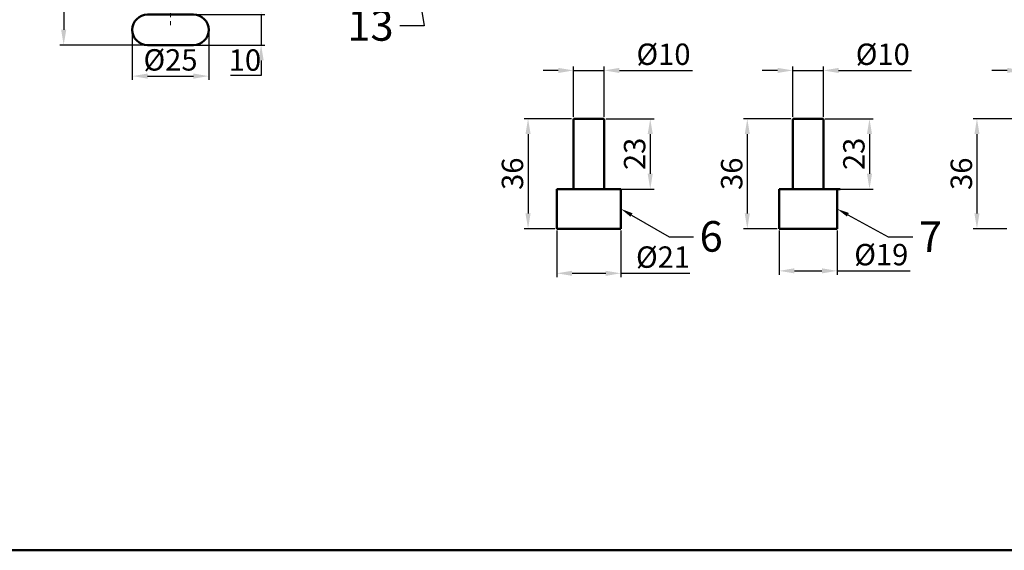
# Model space of a CAD drawing. Units: millimetres. Extents: x 434 to 1535, y -197 to 318.
# Tile 4 of 9: x 726 to 1049, y -197 to -24. Entities that reach past the tile are written whole.
import ezdxf
from ezdxf import colors
from ezdxf.entities.mleader import LeaderData, LeaderLine
from ezdxf.math import Vec2, Vec3

# ---------------------------------------------------------------- set-up
doc = ezdxf.new("R2010")
doc.units = ezdxf.units.MM
doc.header["$LTSCALE"] = 0.4
doc.linetypes.add('CENTER2', pattern=[28.575, 19.05, -3.175, 3.175, -3.175])
for name, color, linetype, lineweight in [('M-CNTR', 1, 'CENTER2', 18), ('M-DIMS', 2, 'Continuous', 25), ('M-OUTL', 7, 'Continuous', 50), ('M-TEXT', 3, 'Continuous', 25)]:
    doc.layers.add(name, color=color, linetype=linetype, lineweight=lineweight)
doc.styles.get("Standard").update_dxf_attribs({"font": 'arial.ttf'})
doc.dimstyles.new('ISO-25', dxfattribs={"dimtxt": 7, "dimasz": 5, "dimexe": 1.25, "dimexo": 0.625, "dimtad": 1, "dimtoh": 1, "dimdec": 0, "dimtxsty": 'Standard', "dimcen": 2.5, "dimadec": 0, "dimazin": 0, "dimtfac": 1, "dimtdec": 0, "dimtmove": 0, "dimatfit": 3, "dimfxl": 1, "dimarcsym": 0})

# ---------------------------------------------------------------- blocks, each defined once
blk = doc.blocks.new('*U48')
at = {"layer": 'M-CNTR', "color": 0, "transparency": 16777216}
blk.add_line((0, 223.89), (0, -74.65), dxfattribs=at)
blk = doc.blocks.new('*D53')
at = {"layer": 'Defpoints', "color": 0, "ltscale": 0.4, "transparency": 16777216}
for p in [(770.74, 232.87), (740.77, -32.13), (770.74, -32.13)]:
    blk.add_point(p, dxfattribs=at)
at = {"layer": 'M-DIMS', "color": 0, "lineweight": -2, "ltscale": 0.4, "transparency": 16777216}
for p, q in [((770.11, 232.87), (739.52, 232.87)), ((740.77, 227.87), (740.77, -27.13)), ((770.11, -32.13), (739.52, -32.13))]:
    blk.add_line(p, q, dxfattribs=at)
at = {"layer": 'M-DIMS', "color": 0, "ltscale": 0.4, "transparency": 16777216}
for points in [[(739.94, 227.87), (741.61, 227.87), (740.77, 232.87)], [(739.94, -27.13), (741.61, -27.13), (740.77, -32.13)]]:
    blk.add_solid(points, dxfattribs=at)
at = {"layer": 'M-DIMS', "color": 0, "ltscale": 0.4, "transparency": 16777216, "insert": (736.57, 100.37), "char_height": 7, "attachment_point": 5, "rotation": 90}
blk.add_mtext('265', dxfattribs=at)
blk = doc.blocks.new('*D54')
at = {"layer": 'Defpoints', "color": 0, "ltscale": 0.4, "transparency": 16777216}
for p in [(763.24, -27.13), (788.24, -27.13), (788.24, -42.28)]:
    blk.add_point(p, dxfattribs=at)
at = {"layer": 'M-DIMS', "color": 0, "lineweight": -2, "ltscale": 0.4, "transparency": 16777216}
for p, q in [((763.24, -27.75), (763.24, -43.53)), ((788.24, -27.75), (788.24, -43.53)), ((768.24, -42.28), (783.24, -42.28))]:
    blk.add_line(p, q, dxfattribs=at)
at = {"layer": 'M-DIMS', "color": 0, "ltscale": 0.4, "transparency": 16777216}
for points in [[(768.24, -41.44), (768.24, -43.11), (763.24, -42.28)], [(783.24, -41.44), (783.24, -43.11), (788.24, -42.28)]]:
    blk.add_solid(points, dxfattribs=at)
at = {"layer": 'M-DIMS', "color": 0, "ltscale": 0.4, "transparency": 16777216, "insert": (775.74, -37.88), "char_height": 7, "attachment_point": 5}
blk.add_mtext('%%C25', dxfattribs=at)
blk = doc.blocks.new('*D68')
at = {"layer": 'Defpoints', "color": 0, "ltscale": 0.4, "transparency": 16777216}
for p in [(775.74, -22.13), (775.74, -32.13), (805.39, -32.13)]:
    blk.add_point(p, dxfattribs=at)
at = {"layer": 'M-DIMS', "color": 0, "lineweight": -2, "ltscale": 0.4, "transparency": 16777216}
for p, q in [((805.39, -17.13), (805.39, -12.13)), ((776.36, -22.13), (806.64, -22.13)), ((805.39, -22.13), (805.39, -32.13)), ((776.36, -32.13), (806.64, -32.13)), ((805.39, -37.13), (805.39, -42.13)), ((805.39, -42.13), (795.42, -42.13))]:
    blk.add_line(p, q, dxfattribs=at)
at = {"layer": 'M-DIMS', "color": 0, "ltscale": 0.4, "transparency": 16777216}
for points in [[(804.55, -17.13), (806.22, -17.13), (805.39, -22.13)], [(804.55, -37.13), (806.22, -37.13), (805.39, -32.13)]]:
    blk.add_solid(points, dxfattribs=at)
at = {"layer": 'M-DIMS', "color": 0, "ltscale": 0.4, "transparency": 16777216, "insert": (800.09, -37.93), "char_height": 7, "attachment_point": 5}
blk.add_mtext('10', dxfattribs=at)
blk = doc.blocks.new('*D111')
at = {"layer": 'Defpoints', "color": 0, "ltscale": 0.4, "transparency": 16777216}
for p in [(917.65, -40.42), (907.65, -56.24), (917.65, -56.24)]:
    blk.add_point(p, dxfattribs=at)
at = {"layer": 'M-DIMS', "color": 0, "lineweight": -2, "ltscale": 0.4, "transparency": 16777216}
for p, q in [((902.65, -40.42), (897.65, -40.42)), ((907.65, -55.61), (907.65, -39.17)), ((907.65, -40.42), (917.65, -40.42)), ((917.65, -55.61), (917.65, -39.17)), ((922.65, -40.42), (946.52, -40.42))]:
    blk.add_line(p, q, dxfattribs=at)
at = {"layer": 'M-DIMS', "color": 0, "ltscale": 0.4, "transparency": 16777216}
for points in [[(902.65, -39.59), (902.65, -41.26), (907.65, -40.42)], [(922.65, -39.59), (922.65, -41.26), (917.65, -40.42)]]:
    blk.add_solid(points, dxfattribs=at)
at = {"layer": 'M-DIMS', "color": 0, "ltscale": 0.4, "transparency": 16777216, "insert": (937.08, -36.03), "char_height": 7, "attachment_point": 5}
blk.add_mtext('%%C10', dxfattribs=at)
blk = doc.blocks.new('*D112')
at = {"layer": 'Defpoints', "color": 0, "ltscale": 0.4, "transparency": 16777216}
for p in [(902.15, -92.24), (923.15, -92.24), (923.15, -106.82)]:
    blk.add_point(p, dxfattribs=at)
at = {"layer": 'M-DIMS', "color": 0, "lineweight": -2, "ltscale": 0.4, "transparency": 16777216}
for p, q in [((902.15, -92.86), (902.15, -108.07)), ((923.15, -92.86), (923.15, -108.07)), ((907.15, -106.82), (918.15, -106.82)), ((923.15, -106.82), (945.69, -106.82))]:
    blk.add_line(p, q, dxfattribs=at)
at = {"layer": 'M-DIMS', "color": 0, "ltscale": 0.4, "transparency": 16777216}
for points in [[(907.15, -105.99), (907.15, -107.66), (902.15, -106.82)], [(918.15, -105.99), (918.15, -107.66), (923.15, -106.82)]]:
    blk.add_solid(points, dxfattribs=at)
at = {"layer": 'M-DIMS', "color": 0, "ltscale": 0.4, "transparency": 16777216, "insert": (936.92, -102.43), "char_height": 7, "attachment_point": 5}
blk.add_mtext('%%C21', dxfattribs=at)
blk = doc.blocks.new('*D113')
at = {"layer": 'Defpoints', "color": 0, "ltscale": 0.4, "transparency": 16777216}
for p in [(917.65, -56.24), (917.65, -79.24), (932.74, -79.24)]:
    blk.add_point(p, dxfattribs=at)
at = {"layer": 'M-DIMS', "color": 0, "lineweight": -2, "ltscale": 0.4, "transparency": 16777216}
for p, q in [((918.27, -56.24), (933.99, -56.24)), ((932.74, -61.24), (932.74, -74.24)), ((918.27, -79.24), (933.99, -79.24))]:
    blk.add_line(p, q, dxfattribs=at)
at = {"layer": 'M-DIMS', "color": 0, "ltscale": 0.4, "transparency": 16777216}
for points in [[(931.9, -61.24), (933.57, -61.24), (932.74, -56.24)], [(931.9, -74.24), (933.57, -74.24), (932.74, -79.24)]]:
    blk.add_solid(points, dxfattribs=at)
at = {"layer": 'M-DIMS', "color": 0, "ltscale": 0.4, "transparency": 16777216, "insert": (928.54, -67.74), "char_height": 7, "attachment_point": 5, "rotation": 90}
blk.add_mtext('23', dxfattribs=at)
blk = doc.blocks.new('*D114')
at = {"layer": 'Defpoints', "color": 0, "ltscale": 0.4, "transparency": 16777216}
for p in [(907.65, -56.24), (892.75, -92.24), (902.15, -92.24)]:
    blk.add_point(p, dxfattribs=at)
at = {"layer": 'M-DIMS', "color": 0, "lineweight": -2, "ltscale": 0.4, "transparency": 16777216}
for p, q in [((907.02, -56.24), (891.5, -56.24)), ((892.75, -61.24), (892.75, -87.24)), ((901.52, -92.24), (891.5, -92.24))]:
    blk.add_line(p, q, dxfattribs=at)
at = {"layer": 'M-DIMS', "color": 0, "ltscale": 0.4, "transparency": 16777216}
for points in [[(891.91, -61.24), (893.58, -61.24), (892.75, -56.24)], [(891.91, -87.24), (893.58, -87.24), (892.75, -92.24)]]:
    blk.add_solid(points, dxfattribs=at)
at = {"layer": 'M-DIMS', "color": 0, "ltscale": 0.4, "transparency": 16777216, "insert": (888.55, -74.24), "char_height": 7, "attachment_point": 5, "rotation": 90}
blk.add_mtext('36', dxfattribs=at)
blk = doc.blocks.new('*D116')
at = {"layer": 'Defpoints', "color": 0, "ltscale": 0.4, "transparency": 16777216}
for p in [(989.4, -40.42), (979.4, -56.24), (989.4, -56.24)]:
    blk.add_point(p, dxfattribs=at)
at = {"layer": 'M-DIMS', "color": 0, "lineweight": -2, "ltscale": 0.4, "transparency": 16777216}
for p, q in [((974.4, -40.42), (969.4, -40.42)), ((979.4, -55.61), (979.4, -39.17)), ((979.4, -40.42), (989.4, -40.42)), ((989.4, -55.61), (989.4, -39.17)), ((994.4, -40.42), (1018.27, -40.42))]:
    blk.add_line(p, q, dxfattribs=at)
at = {"layer": 'M-DIMS', "color": 0, "ltscale": 0.4, "transparency": 16777216}
for points in [[(974.4, -39.59), (974.4, -41.26), (979.4, -40.42)], [(994.4, -39.59), (994.4, -41.26), (989.4, -40.42)]]:
    blk.add_solid(points, dxfattribs=at)
at = {"layer": 'M-DIMS', "color": 0, "ltscale": 0.4, "transparency": 16777216, "insert": (1008.84, -36.03), "char_height": 7, "attachment_point": 5}
blk.add_mtext('%%C10', dxfattribs=at)
blk = doc.blocks.new('*D117')
at = {"layer": 'Defpoints', "color": 0, "ltscale": 0.4, "transparency": 16777216}
for p in [(989.4, -56.24), (989.4, -79.24), (1004.49, -79.24)]:
    blk.add_point(p, dxfattribs=at)
at = {"layer": 'M-DIMS', "color": 0, "lineweight": -2, "ltscale": 0.4, "transparency": 16777216}
for p, q in [((990.03, -56.24), (1005.74, -56.24)), ((1004.49, -61.24), (1004.49, -74.24)), ((990.03, -79.24), (1005.74, -79.24))]:
    blk.add_line(p, q, dxfattribs=at)
at = {"layer": 'M-DIMS', "color": 0, "ltscale": 0.4, "transparency": 16777216}
for points in [[(1003.66, -61.24), (1005.32, -61.24), (1004.49, -56.24)], [(1003.66, -74.24), (1005.32, -74.24), (1004.49, -79.24)]]:
    blk.add_solid(points, dxfattribs=at)
at = {"layer": 'M-DIMS', "color": 0, "ltscale": 0.4, "transparency": 16777216, "insert": (1000.29, -67.74), "char_height": 7, "attachment_point": 5, "rotation": 90}
blk.add_mtext('23', dxfattribs=at)
blk = doc.blocks.new('*D115')
at = {"layer": 'Defpoints', "color": 0, "ltscale": 0.4, "transparency": 16777216}
for p in [(979.4, -56.24), (964.5, -92.24), (974.9, -92.24)]:
    blk.add_point(p, dxfattribs=at)
at = {"layer": 'M-DIMS', "color": 0, "lineweight": -2, "ltscale": 0.4, "transparency": 16777216}
for p, q in [((978.78, -56.24), (963.25, -56.24)), ((964.5, -61.24), (964.5, -87.24)), ((974.28, -92.24), (963.25, -92.24))]:
    blk.add_line(p, q, dxfattribs=at)
at = {"layer": 'M-DIMS', "color": 0, "ltscale": 0.4, "transparency": 16777216}
for points in [[(963.67, -61.24), (965.33, -61.24), (964.5, -56.24)], [(963.67, -87.24), (965.33, -87.24), (964.5, -92.24)]]:
    blk.add_solid(points, dxfattribs=at)
at = {"layer": 'M-DIMS', "color": 0, "ltscale": 0.4, "transparency": 16777216, "insert": (960.3, -74.24), "char_height": 7, "attachment_point": 5, "rotation": 90}
blk.add_mtext('36', dxfattribs=at)
blk = doc.blocks.new('*D118')
at = {"layer": 'Defpoints', "color": 0, "ltscale": 0.4, "transparency": 16777216}
for p in [(974.9, -92.24), (993.9, -92.24), (993.9, -106.02)]:
    blk.add_point(p, dxfattribs=at)
at = {"layer": 'M-DIMS', "color": 0, "lineweight": -2, "ltscale": 0.4, "transparency": 16777216}
for p, q in [((974.9, -92.86), (974.9, -107.27)), ((993.9, -92.86), (993.9, -107.27)), ((979.9, -106.02), (988.9, -106.02)), ((993.9, -106.02), (1017.81, -106.02))]:
    blk.add_line(p, q, dxfattribs=at)
at = {"layer": 'M-DIMS', "color": 0, "ltscale": 0.4, "transparency": 16777216}
for points in [[(979.9, -105.18), (979.9, -106.85), (974.9, -106.02)], [(988.9, -105.18), (988.9, -106.85), (993.9, -106.02)]]:
    blk.add_solid(points, dxfattribs=at)
at = {"layer": 'M-DIMS', "color": 0, "ltscale": 0.4, "transparency": 16777216, "insert": (1008.35, -101.62), "char_height": 7, "attachment_point": 5}
blk.add_mtext('%%C19', dxfattribs=at)
blk = doc.blocks.new('*D120')
at = {"layer": 'Defpoints', "color": 0, "ltscale": 0.4, "transparency": 16777216}
for p in [(1064.56, -40.42), (1054.56, -56.24), (1064.56, -56.24)]:
    blk.add_point(p, dxfattribs=at)
at = {"layer": 'M-DIMS', "color": 0, "lineweight": -2, "ltscale": 0.4, "transparency": 16777216}
for p, q in [((1049.56, -40.42), (1044.56, -40.42)), ((1054.56, -55.61), (1054.56, -39.17)), ((1054.56, -40.42), (1064.56, -40.42)), ((1064.56, -55.61), (1064.56, -39.17)), ((1069.56, -40.42), (1093.43, -40.42))]:
    blk.add_line(p, q, dxfattribs=at)
at = {"layer": 'M-DIMS', "color": 0, "ltscale": 0.4, "transparency": 16777216}
for points in [[(1049.56, -39.59), (1049.56, -41.26), (1054.56, -40.42)], [(1069.56, -39.59), (1069.56, -41.26), (1064.56, -40.42)]]:
    blk.add_solid(points, dxfattribs=at)
at = {"layer": 'M-DIMS', "color": 0, "ltscale": 0.4, "transparency": 16777216, "insert": (1083.99, -36.03), "char_height": 7, "attachment_point": 5}
blk.add_mtext('%%C10', dxfattribs=at)
blk = doc.blocks.new('*D119')
at = {"layer": 'Defpoints', "color": 0, "ltscale": 0.4, "transparency": 16777216}
for p in [(1054.56, -56.24), (1039.66, -92.24), (1050.06, -92.24)]:
    blk.add_point(p, dxfattribs=at)
at = {"layer": 'M-DIMS', "color": 0, "lineweight": -2, "ltscale": 0.4, "transparency": 16777216}
for p, q in [((1053.93, -56.24), (1038.41, -56.24)), ((1039.66, -61.24), (1039.66, -87.24)), ((1049.43, -92.24), (1038.41, -92.24))]:
    blk.add_line(p, q, dxfattribs=at)
at = {"layer": 'M-DIMS', "color": 0, "ltscale": 0.4, "transparency": 16777216}
for points in [[(1038.83, -61.24), (1040.49, -61.24), (1039.66, -56.24)], [(1038.83, -87.24), (1040.49, -87.24), (1039.66, -92.24)]]:
    blk.add_solid(points, dxfattribs=at)
at = {"layer": 'M-DIMS', "color": 0, "ltscale": 0.4, "transparency": 16777216, "insert": (1035.46, -74.24), "char_height": 7, "attachment_point": 5, "rotation": 90}
blk.add_mtext('36', dxfattribs=at)

msp = doc.modelspace()

# ---------------------------------------------------------------- linework, layer by layer
at = {"layer": 'M-OUTL', "ltscale": 0.4}
for p, q in [((917.65, -56.24), (907.65, -56.24)), ((907.65, -56.24), (907.65, -79.24)), ((917.65, -79.24), (917.65, -56.24)), ((989.4, -56.24), (979.4, -56.24)), ((979.4, -56.24), (979.4, -79.24)), ((989.4, -79.24), (989.4, -56.24)), ((923.15, -79.24), (902.15, -79.24)), ((902.15, -79.24), (902.15, -92.24)), ((923.15, -92.24), (923.15, -79.24)), ((994.9, -79.24), (974.9, -79.24)), ((974.9, -79.24), (974.9, -92.24)), ((993.9, -92.24), (993.9, -79.24)), ((902.15, -92.24), (923.15, -92.24)), ((974.9, -92.24), (993.9, -92.24))]:
    msp.add_line(p, q, dxfattribs=at)
msp.add_lwpolyline([(434.2, 318.45), (1535.47, 318.45), (1535.47, -197.48), (434.2, -197.48)], close=True, dxfattribs=at)
msp.add_lwpolyline([(768.24, -22.13, 1), (768.24, -32.13), (783.24, -32.13, 1), (783.24, -22.13)], format="xyb", close=True, dxfattribs=at)

# ---------------------------------------------------------------- block references
at = {"layer": 'M-CNTR'}
msp.add_blockref('*U48', (775.74, 49.02), dxfattribs=at)

# ---------------------------------------------------------------- dimensions: what is measured, and where the dimension line sits
at = {"layer": 'M-DIMS', "ltscale": 0.4}
for base, p1, p2, picture, middle in [((740.77, -32.13), (770.74, 232.87), (770.74, -32.13), '*D53', (736.57, 100.37)), ((805.39, -32.13), (775.74, -22.13), (775.74, -32.13), '*D68', (800.09, -37.93)), ((892.75, -92.24), (907.65, -56.24), (902.15, -92.24), '*D114', (888.55, -74.24)), ((932.74, -79.24), (917.65, -56.24), (917.65, -79.24), '*D113', (928.54, -67.74)), ((964.5, -92.24), (979.4, -56.24), (974.9, -92.24), '*D115', (960.3, -74.24)), ((1004.49, -79.24), (989.4, -56.24), (989.4, -79.24), '*D117', (1000.29, -67.74)), ((1039.66, -92.24), (1054.56, -56.24), (1050.06, -92.24), '*D119', (1035.46, -74.24))]:
    dim = msp.add_linear_dim(base=base, p1=p1, p2=p2, angle=90, dimstyle='ISO-25', override={"dimclrd": 0, "dimclre": 0, "dimclrt": 0}, dxfattribs=at)
    dim.commit()
    dim.dimension.update_dxf_attribs({"geometry": picture, "text_midpoint": middle})
for base, p1, p2, picture, middle in [((788.24, -42.28), (763.24, -27.13), (788.24, -27.13), '*D54', (775.74, -37.88)), ((917.65, -40.42), (907.65, -56.24), (917.65, -56.24), '*D111', (937.08, -36.03)), ((989.4, -40.42), (979.4, -56.24), (989.4, -56.24), '*D116', (1008.84, -36.03)), ((1064.56, -40.42), (1054.56, -56.24), (1064.56, -56.24), '*D120', (1083.99, -36.03))]:
    dim = msp.add_linear_dim(base=base, p1=p1, p2=p2, text='%%C<>', dimstyle='ISO-25', override={"dimclrd": 0, "dimclre": 0, "dimclrt": 0}, dxfattribs=at)
    dim.commit()
    dim.dimension.update_dxf_attribs({"geometry": picture, "text_midpoint": middle})
for base, p1, p2, picture, middle in [((923.15, -106.82), (902.15, -92.24), (923.15, -92.24), '*D112', (936.92, -106.82)), ((993.9, -106.02), (974.9, -92.24), (993.9, -92.24), '*D118', (1008.35, -106.02))]:
    dim = msp.add_linear_dim(base=base, p1=p1, p2=p2, text='%%C<>', dimstyle='ISO-25', override={"dimclrd": 0, "dimclre": 0, "dimclrt": 0}, dxfattribs=at)
    dim.commit()
    dim.dimension.update_dxf_attribs({"geometry": picture, "text_midpoint": middle, "dimtype": 160})

# ---------------------------------------------------------------- leaders
at = {"layer": 'M-TEXT', "ltscale": 0.4}
ml = msp.add_multileader_mtext('Standard', dxfattribs=at)
ml.set_content('13', color=256)
ml.set_leader_properties()
ml.build(insert=Vec2(0, 0))
ctx = ml.context
ctx.base_point, ctx.char_height, ctx.plane_origin = Vec3(833.37, -25.8), 10, Vec3(855.91, -8.31)
ctx.text_align_type = 2
notes = []
notes.append((ctx, [(0, (1, 1, 0), (858.75, -25.8), (-1, 0), 8, [(0, [(855.91, -8.31)], 0, [])])]))
ctx.mtext.insert, ctx.mtext.alignment, ctx.mtext.flow_direction = Vec3(848.75, -20.71), 3, 5
ml = msp.add_multileader_mtext('Standard', dxfattribs=at)
ml.set_content('6', color=256)
ml.set_leader_properties()
ml.build(insert=Vec2(0, 0))
ctx = ml.context
ctx.base_point, ctx.char_height, ctx.plane_origin = Vec3(946.89, -94.83), 10, Vec3(923.15, -85.74)
notes.append((ctx, [(0, (1, 1, 0), (938.89, -94.83), (1, 0), 8, [(0, [(923.15, -85.74)], 0, [])])]))
ctx.mtext.insert, ctx.mtext.flow_direction = Vec3(948.89, -89.74), 5
ml = msp.add_multileader_mtext('Standard', dxfattribs=at)
ml.set_content('7', color=256)
ml.set_leader_properties()
ml.build(insert=Vec2(0, 0))
ctx = ml.context
ctx.base_point, ctx.char_height, ctx.plane_origin = Vec3(1018.65, -94.83), 10, Vec3(994.9, -85.74)
notes.append((ctx, [(0, (1, 1, 0), (1010.65, -94.83), (1, 0), 8, [(0, [(993.9, -85.74)], 0, [])])]))
ctx.mtext.insert, ctx.mtext.flow_direction = Vec3(1020.65, -89.83), 5
for ctx, leaders in notes:
    for number, flags, end, landing, length, lines in leaders:
        leader = LeaderData()
        leader.index, (leader.has_last_leader_line, leader.has_dogleg_vector, leader.attachment_direction) = number, flags
        leader.last_leader_point, leader.dogleg_vector, leader.dogleg_length = Vec3(end), Vec3(landing), length
        for number, points, colour, breaks in lines:
            line = LeaderLine()
            line.index, line.vertices, line.color, line.breaks = number, Vec3.list(points), colors.encode_raw_color(colour), breaks
            leader.lines.append(line)
        ctx.leaders.append(leader)

doc.saveas('drawing.dxf')
